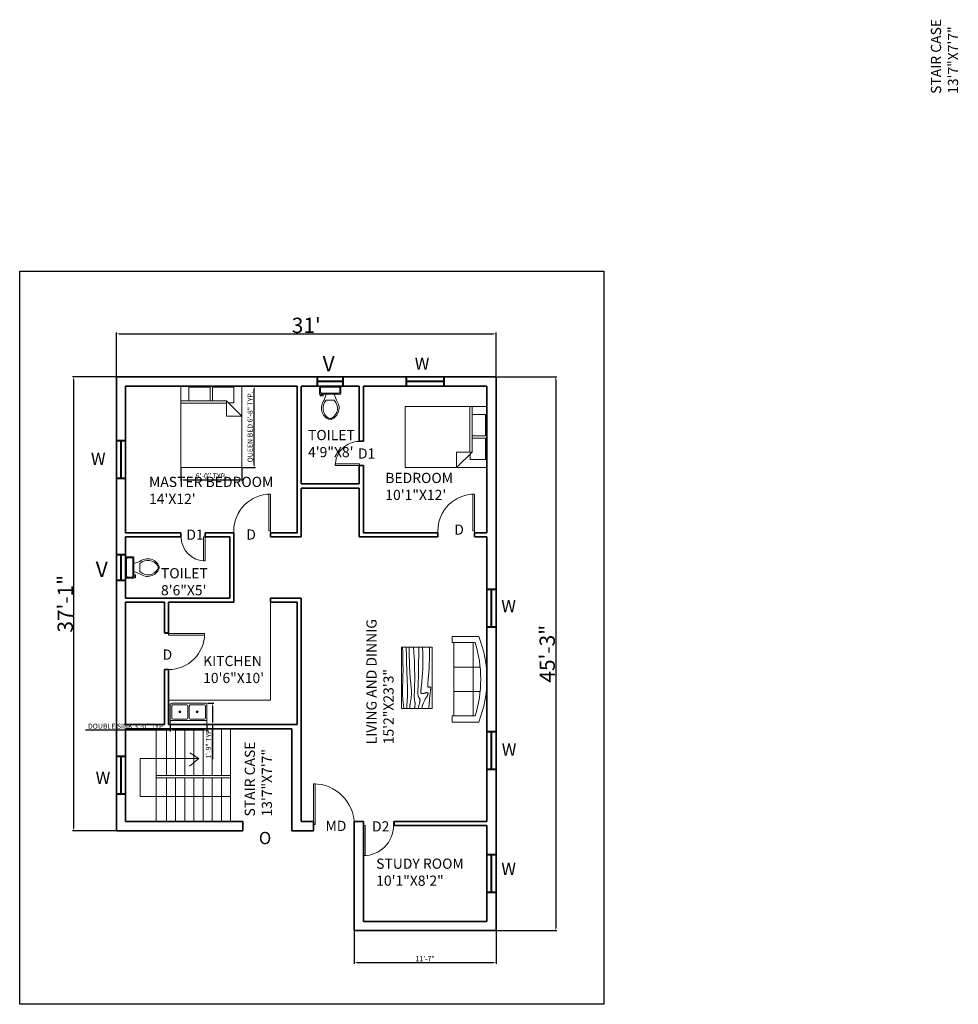
# Model space of a CAD drawing. Units: inches. Extents: x 1662 to 23131, y 1265 to 19127.
# Tile 3 of 26: x 1662 to 2582, y 4561 to 5526. Entities that reach past the tile are written whole.
import ezdxf

# ---------------------------------------------------------------- set-up
doc = ezdxf.new("R2010")
doc.units = ezdxf.units.IN
for name, color, linetype, lineweight in [('A-ANNO-DIMS', 4, 'Continuous', 18), ('A-ANNO-IDEN', 7, 'Continuous', 18), ('A-ANNO-TTLB', 7, 'Continuous', 25), ('A-AREA-IDEN', 7, 'Continuous', 18), ('A-DOOR', 3, 'Continuous', 18), ('A-FLOR-CASE', 8, 'Continuous', 18), ('A-FLOR-FIXT', 9, 'Continuous', 18), ('A-FLOR-STRS', 7, 'Continuous', 18), ('A-FURN', 8, 'Continuous', 18), ('A-GLAZ', 4, 'Continuous', 18), ('A-WALL', 7, 'Continuous', 35)]:
    doc.layers.add(name, color=color, linetype=linetype, lineweight=lineweight)
doc.styles.get("Standard").update_dxf_attribs({"font": 'arial.ttf'})
doc.dimstyles.new('ISO-25', dxfattribs={"dimtxt": 5, "dimasz": 2.5, "dimexe": 1.25, "dimexo": 0.625, "dimtad": 1, "dimlunit": 3, "dimtxsty": 'Standard', "dimcen": 2.5, "dimadec": 0, "dimazin": 0, "dimtfac": 1, "dimtmove": 0, "dimatfit": 3, "dimfxl": 1, "dimarcsym": 0})

# ---------------------------------------------------------------- blocks, each defined once
blk = doc.blocks.new('*U33')
for p, q in [((0, 0), (0, -6)), ((40, 0), (40, -6))]:
    blk.add_line(p, q)
blk.add_lwpolyline([(0, 0), (0, 40), (1.75, 40), (1.75, 0)], close=True)
blk.add_arc((0, 0), 40, 0, 90)
blk = doc.blocks.new('*U25')
for p, q in [((-750, 0), (-750, -100)), ((0, 0), (0, -100))]:
    blk.add_line(p, q)
blk.add_lwpolyline([(0, 0), (0, 750), (-43.75, 750), (-43.75, 0)], close=True)
blk.add_arc((0, 0), 750, 90, 180)
blk = doc.blocks.new('*U34')
for p, q in [((0, 0), (0, -6)), ((-36, 0), (-36, -6))]:
    blk.add_line(p, q)
blk.add_lwpolyline([(0, 0), (0, 36), (-1.75, 36), (-1.75, 0)], close=True)
blk.add_arc((0, 0), 36, 90, 180)
blk = doc.blocks.new('*U35')
for p, q in [((0, 0), (0, -100)), ((600, 0), (600, -100))]:
    blk.add_line(p, q)
blk.add_lwpolyline([(0, 0), (0, 600), (43.75, 600), (43.75, 0)], close=True)
blk.add_arc((0, 0), 600, 0, 90)
blk = doc.blocks.new('*U36')
for p, q in [((-900, 0), (-900, 100)), ((0, 0), (0, 100))]:
    blk.add_line(p, q)
blk.add_lwpolyline([(0, 0), (0, -900), (-43.75, -900), (-43.75, 0)], close=True)
blk.add_arc((0, 0), 900, 180, 270)
blk = doc.blocks.new('Bed - Queen')
for p, q in [((0, -80.00003), (0, 0)), ((0, 0), (59.99999, 0)), ((59.99999, 0), (59.99999, -80.00003)), ((7.99999, -1.2), (28.79998, -1.2)), ((7.99999, -14.4), (7.99999, -1.2)), ((28.79998, -1.2), (28.79998, -14.4)), ((31.19999, -1.2), (51.99999, -1.2)), ((31.19999, -14.4), (31.19999, -1.2)), ((51.99999, -1.2), (51.99999, -16.4)), ((0, -14.4), (44.8, -14.4)), ((44.8, -16.8), (0, -16.8)), ((59.99999, -29.6), (44.8, -14.4)), ((44.8, -14.4), (44.8, -29.6)), ((51.99999, -16.4), (46.79936, -16.4)), ((44.8, -29.6), (59.99999, -29.6)), ((59.99999, -80.00003), (0, -80.00003))]:
    blk.add_line(p, q)
blk = doc.blocks.new('Sink-double - 36 in top')
for p, q in [((-18, -4), (18, -4)), ((-0.75, -18.5), (-0.75, -6.5)), ((0.75, -6.5), (0.75, -18.5))]:
    blk.add_line(p, q)
for points in [[(-16.5, 0), (16.5, 0)], [(-18, -19.5), (-18, -1.5)], [(-16.5, -18.5), (-16.5, -6.5)], [(-15.5, -5.5), (-1.75, -5.5)], [(1.75, -5.5), (15.5, -5.5)], [(16.5, -6.5), (16.5, -18.5)], [(18, -1.5), (18, -19.5)], [(16.5, -21), (-16.5, -21)], [(-1.75, -19.5), (-15.5, -19.5)], [(15.5, -19.5), (1.75, -19.5)]]:
    blk.add_lwpolyline(points)
for centre, radius in [((-8.5, -12.5), 1), ((-8.5, -12.5), 0.5), ((8.5, -12.5), 1), ((8.5, -12.5), 0.5)]:
    blk.add_circle(centre, radius)
for centre, radius, start, end in [((-16.5, -1.5), 1.5, 90, 180), ((16.5, -1.5), 1.5, 0, 90), ((-15.5, -6.5), 1, 90, 180), ((-1.75, -6.5), 1, 0, 90), ((1.75, -6.5), 1, 90, 180), ((15.5, -6.5), 1, 0, 90), ((-15.5, -18.5), 1, 180, 270), ((-1.75, -18.5), 1, 270, 0), ((1.75, -18.5), 1, 180, 270), ((15.5, -18.5), 1, 270, 0), ((-16.5, -19.5), 1.5, 180, 270), ((16.5, -19.5), 1.5, 270, 0)]:
    blk.add_arc(centre, radius, start, end)
blk = doc.blocks.new('Sofa - Roundback 7 ft.')
for p, q in [((-12.00002, -32.4421), (-12.00003, -6.5971)), ((11.99997, -32.4421), (11.99998, -6.5971)), ((-36.000027, -34), (-36.000027, -11.4696)), ((-35.999844, -13.3819), (35.9998, -13.3819)), ((35.99998, -34), (35.99998, -11.4696)), ((-36.000027, -32.4421), (35.99998, -32.4421))]:
    blk.add_line(p, q)
for points in [[(-36.000027, -34), (-42.000027, -34), (-42.000027, -8)], [(41.99998, -8), (41.99998, -34), (35.99998, -34)]]:
    blk.add_lwpolyline(points)
for centre, radius, start, end in [((0, -114.25), 114.25, 68.43141, 111.5686), ((-0.00001, -127.1968), 121.1968, 72.72033, 107.2797)]:
    blk.add_arc(centre, radius, start, end)
blk = doc.blocks.new('Table - Rectangular Woodgrain 60 x 30 in.')
for p, q in [((0, 0), (0, -30)), ((60, 0), (0, 0)), ((60, -30), (60, 0)), ((0, -30), (60, -30))]:
    blk.add_line(p, q)
for points in [[(0, -2.4), (4.8155, -2.418), (9.0302, -2.4688), (12.709, -2.5477), (15.9167, -2.65), (18.7181, -2.7711), (21.1781, -2.9063), (23.3616, -3.0508), (25.3333, -3.2), (27.1477, -3.3495), (28.8172, -3.4958), (30.3437, -3.636), (31.7291, -3.7667), (32.9756, -3.8849), (34.0849, -3.9875), (35.059, -4.0714), (35.9, -4.1334), (36.6114, -4.1711), (37.2041, -4.1854), (37.6906, -4.1779), (38.0833, -4.15), (38.3948, -4.1034), (38.6375, -4.0396), (38.8239, -3.9602), (38.9666, -3.8667), (39.0764, -3.7608), (39.1573, -3.6448), (39.2116, -3.521), (39.2416, -3.3917), (39.2498, -3.2593), (39.2385, -3.1261), (39.21, -2.9944), (39.1666, -2.8667), (39.111, -2.7447), (39.0468, -2.6281), (38.978, -2.5163), (38.9083, -2.4083), (38.8418, -2.3035), (38.7823, -2.201), (38.7337, -2.1001), (38.7, -2), (38.6844, -1.9003), (38.6875, -1.8021), (38.7094, -1.707), (38.75, -1.6167), (38.8094, -1.5326), (38.8875, -1.4563), (38.9844, -1.3893), (39.1, -1.3333), (39.2351, -1.2896), (39.3937, -1.2583), (39.5804, -1.2396), (39.8, -1.2333), (40.057, -1.2396), (40.3562, -1.2583), (40.7023, -1.2896), (41.1, -1.3333), (41.5547, -1.3895), (42.0755, -1.4573), (42.6721, -1.5361), (43.3542, -1.625), (44.1316, -1.7233), (45.014, -1.8302), (46.0114, -1.9449), (47.1333, -2.0667), (48.3862, -2.1947), (49.7625, -2.3281), (51.2513, -2.4663), (52.8416, -2.6083), (54.5226, -2.7535), (56.2833, -2.9011), (58.1127, -3.0501), (60, -3.2)], [(0, -9.2), (6.5759, -9.0858), (11.9385, -9.0365), (16.2527, -9.0418), (19.6833, -9.0917), (22.3952, -9.1759), (24.5531, -9.2844), (26.322, -9.4069), (27.8666, -9.5333), (29.3241, -9.6553), (30.7203, -9.7719), (32.0532, -9.8837), (33.3208, -9.9917), (34.5213, -10.0965), (35.6526, -10.199), (36.7128, -10.2999), (37.7, -10.4), (38.6129, -10.4996), (39.4531, -10.5969), (40.223, -10.6895), (40.925, -10.775), (41.5613, -10.8512), (42.1344, -10.9156), (42.6465, -10.966), (43.1, -11), (43.4976, -11.0158), (43.8437, -11.0136), (44.143, -10.9942), (44.4, -10.9583), (44.6195, -10.9069), (44.8062, -10.8406), (44.9648, -10.7603), (45.1, -10.6667), (45.2155, -10.5598), (45.3114, -10.4365), (45.3871, -10.2929), (45.4416, -10.125), (45.4743, -9.929), (45.4844, -9.7011), (45.4709, -9.4371), (45.4333, -9.1333), (45.3716, -8.7883), (45.2896, -8.4104), (45.1919, -8.0107), (45.0833, -7.6), (44.9685, -7.1893), (44.8521, -6.7896), (44.7388, -6.4117), (44.6333, -6.0667), (44.54, -5.7628), (44.4614, -5.4979), (44.4001, -5.2675), (44.3583, -5.0667), (44.3384, -4.8909), (44.3427, -4.7354), (44.3736, -4.5956), (44.4333, -4.4667), (44.5236, -4.3453), (44.6427, -4.2333), (44.7884, -4.1339), (44.9583, -4.05), (45.1501, -3.9849), (45.3614, -3.9417), (45.59, -3.9234), (45.8333, -3.9333), (46.0915, -3.9749), (46.3734, -4.0531), (46.6906, -4.1736), (47.0542, -4.3417), (47.4756, -4.5629), (47.9661, -4.8427), (48.5372, -5.1866), (49.2, -5.6), (49.9676, -6.0844), (50.8594, -6.625), (51.8965, -7.2031), (53.1, -7.8), (54.491, -8.3969), (56.0906, -8.975), (57.9199, -9.5156), (60, -10)], [(0, -12.8), (5.1847, -12.9322), (9.6213, -13.0323), (13.3963, -13.1059), (16.5958, -13.1583), (19.3063, -13.1952), (21.614, -13.2219), (23.6054, -13.2439), (25.3666, -13.2667), (26.9728, -13.2947), (28.4531, -13.3281), (29.8256, -13.3663), (31.1083, -13.4083), (32.3191, -13.4535), (33.476, -13.501), (34.597, -13.5501), (35.7, -13.6), (36.7984, -13.6497), (37.8875, -13.6979), (38.9578, -13.743), (40, -13.7833), (41.0047, -13.8174), (41.9625, -13.8438), (42.864, -13.8607), (43.7, -13.8667), (44.4631, -13.8604), (45.1552, -13.8417), (45.7801, -13.8104), (46.3416, -13.7667), (46.8439, -13.7104), (47.2906, -13.6417), (47.6858, -13.5604), (48.0333, -13.4667), (48.3375, -13.3608), (48.6042, -13.2448), (48.8396, -13.121), (49.05, -12.9917), (49.2417, -12.8593), (49.4208, -12.7261), (49.5937, -12.5944), (49.7667, -12.4667), (49.9452, -12.3451), (50.1323, -12.2313), (50.3303, -12.1268), (50.5416, -12.0333), (50.7686, -11.9524), (51.0135, -11.8854), (51.2788, -11.8341), (51.5666, -11.8), (51.8785, -11.7843), (52.2116, -11.7865), (52.562, -11.8059), (52.926, -11.8417), (53.2998, -11.8931), (53.6795, -11.9594), (54.0614, -12.0397), (54.4416, -12.1333), (54.8223, -12.2401), (55.2293, -12.3625), (55.6942, -12.5037), (56.2489, -12.6667), (56.9251, -12.8547), (57.7545, -13.0708), (58.7689, -13.3182), (60, -13.6)], [(0, -18), (5.124, -17.7273), (9.6609, -17.5057), (13.6705, -17.3303), (17.2125, -17.1958), (20.3467, -17.0973), (23.1328, -17.0297), (25.6307, -16.9878), (27.9, -16.9667), (29.9928, -16.9617), (31.9302, -16.9703), (33.7254, -16.9907), (35.3917, -17.0208), (36.9423, -17.0588), (38.3906, -17.1026), (39.7499, -17.1503), (41.0333, -17.2), (42.2519, -17.2496), (43.4073, -17.2969), (44.4986, -17.3395), (45.525, -17.375), (46.4858, -17.4012), (47.3802, -17.4156), (48.2074, -17.416), (48.9667, -17.4), (49.6583, -17.3662), (50.2872, -17.3167), (50.8595, -17.2547), (51.3812, -17.1833), (51.8584, -17.1057), (52.2971, -17.025), (52.7034, -16.9443), (53.0833, -16.8667), (53.443, -16.7951), (53.789, -16.7313), (54.128, -16.6768), (54.4666, -16.6334), (54.8115, -16.6024), (55.1693, -16.5854), (55.5465, -16.5841), (55.95, -16.6), (56.3828, -16.6337), (56.8346, -16.6823), (57.2915, -16.7418), (57.7396, -16.8084), (58.165, -16.878), (58.5539, -16.9469), (58.8924, -17.0111), (59.1666, -17.0667), (59.3679, -17.1107), (59.5078, -17.1438), (59.6032, -17.1675), (59.6708, -17.1833), (59.7275, -17.193), (59.7901, -17.1979), (59.8753, -17.1998), (60, -17.2)], [(0, -22.4), (8.0098, -22.2501), (14.4094, -22.1011), (19.4168, -21.9535), (23.25, -21.8083), (26.1269, -21.6663), (28.2656, -21.5281), (29.884, -21.3947), (31.2, -21.2667), (32.3967, -21.1448), (33.5172, -21.0292), (34.5697, -20.9198), (35.5625, -20.8167), (36.5037, -20.7198), (37.4015, -20.6292), (38.2642, -20.5448), (39.1, -20.4667), (39.9164, -20.3951), (40.7187, -20.3313), (41.5117, -20.2768), (42.3, -20.2333), (43.0883, -20.2024), (43.8812, -20.1854), (44.6836, -20.1841), (45.5, -20.2), (46.3328, -20.234), (47.1747, -20.2844), (48.0163, -20.3488), (48.8479, -20.425), (49.66, -20.5106), (50.4429, -20.6031), (51.1872, -20.7004), (51.8833, -20.8), (52.5246, -20.8999), (53.1166, -20.9995), (53.6681, -21.0983), (54.1875, -21.1958), (54.6834, -21.2919), (55.1646, -21.3859), (55.6394, -21.4777), (56.1167, -21.5667), (56.6028, -21.6515), (57.0961, -21.7266), (57.5929, -21.7852), (58.0896, -21.8208), (58.5823, -21.8268), (59.0674, -21.7964), (59.5412, -21.723), (60, -21.6)], [(0, -25.2), (8.6355, -25.0504), (15.7026, -24.9031), (21.4049, -24.7606), (25.9458, -24.625), (29.529, -24.4988), (32.3578, -24.3844), (34.6359, -24.284), (36.5667, -24.2), (38.3213, -24.1341), (39.9417, -24.0854), (41.437, -24.0523), (42.8167, -24.0333), (44.0901, -24.0268), (45.2667, -24.0313), (46.3557, -24.0451), (47.3667, -24.0667), (48.309, -24.0947), (49.1928, -24.1287), (50.0284, -24.168), (50.826, -24.2125), (51.5959, -24.2617), (52.3483, -24.3151), (53.0935, -24.3725), (53.8417, -24.4334), (54.6009, -24.497), (55.3699, -24.561), (56.1454, -24.6226), (56.9239, -24.6792), (57.7021, -24.7279), (58.4764, -24.7662), (59.2435, -24.7911), (60, -24.8)], [(0, -28.8), (5.6867, -28.6681), (10.45, -28.5698), (14.407, -28.5012), (17.675, -28.4584), (20.3711, -28.4374), (22.6125, -28.4344), (24.5164, -28.4455), (26.2, -28.4667), (27.762, -28.4947), (29.2276, -28.5281), (30.6033, -28.5663), (31.8958, -28.6084), (33.1118, -28.6535), (34.2578, -28.7011), (35.3405, -28.7501), (36.3666, -28.8), (37.3443, -28.8497), (38.288, -28.8974), (39.2137, -28.9412), (40.1375, -28.9792), (41.0753, -29.0093), (42.0432, -29.0297), (43.0572, -29.0384), (44.1333, -29.0333), (45.2936, -29.0114), (46.5843, -28.9641), (48.0579, -28.8816), (49.7666, -28.7542), (51.7629, -28.5721), (54.0989, -28.3255), (56.8272, -28.0048), (60, -27.6)]]:
    blk.add_lwpolyline(points)
blk = doc.blocks.new('Toilet - top')
for p, q in [((-10, -8.5), (-8, -8.5)), ((-10, -9.5), (-10, -8.5)), ((-7, -9.5), (-10, -9.5)), ((-8, -8.5), (-8, -8)), ((-7, -8), (-7, -9.5)), ((-4, -8), (-6, -14)), ((4, -8), (6, -14)), ((9.5, -6), (9.5, -2)), ((4, -14), (-4, -14))]:
    blk.add_line(p, q)
blk.add_lwpolyline([(10.5, -8), (10.5, 0), (-10.5, 0), (-10.5, -8)], close=True)
for points in [[(-9.5, -2), (-9.5, -6)], [(8.5, -1), (-8.5, -1)], [(-8.5, -7), (8.5, -7)]]:
    blk.add_lwpolyline(points)
for centre, radius, start, end in [((-8.62, -1.88), 0.884, 81.8699, 188.1301), ((-8.62, -6.12), 0.884, 171.8699, 278.1301), ((8.62, -1.88), 0.884, 351.8699, 98.1301), ((8.62, -6.12), 0.884, 261.8699, 8.1301), ((3.52, -21.58), 12.17, 141.46911, 247.97143), ((4.2, -21.82), 11.33, 136.36773, 238.94682), ((-3.52, -21.58), 12.17, 292.02843, 38.53071), ((-4.2, -21.82), 11.33, 301.05301, 43.63209), ((0, -27.88), 4, 245.73182, 294.26817), ((0, -29), 4, 254.86053, 285.13947)]:
    blk.add_arc(centre, radius, start, end)
blk = doc.blocks.new('*D37')
at = {"layer": 'A-ANNO-DIMS', "color": 0, "lineweight": -2, "transparency": 16777216}
for p, q in [((1757.16, 5176.65), (1757.16, 5219.46)), ((1759.66, 5218.21), (2126.66, 5218.21)), ((2129.16, 5176.65), (2129.16, 5219.46))]:
    blk.add_line(p, q, dxfattribs=at)
at = {"layer": 'A-ANNO-DIMS', "color": 0, "transparency": 16777216}
for points in [[(1759.66, 5218.63), (1759.66, 5217.79), (1757.16, 5218.21)], [(2126.66, 5218.63), (2126.66, 5217.79), (2129.16, 5218.21)]]:
    blk.add_solid(points, dxfattribs=at)
at = {"layer": 'Defpoints', "color": 0, "transparency": 16777216}
for p in [(2129.16, 5218.21), (1757.16, 5176.03), (2129.16, 5176.03)]:
    blk.add_point(p, dxfattribs=at)
at = {"layer": 'A-ANNO-DIMS', "color": 0, "transparency": 16777216, "insert": (1943.16, 5226.5), "char_height": 5, "attachment_point": 5}
blk.add_mtext("{\\H3x;31'}", dxfattribs=at)
blk = doc.blocks.new('*D38')
at = {"layer": 'A-ANNO-DIMS', "color": 0, "lineweight": -2, "transparency": 16777216}
for p, q in [((2129.79, 5176.03), (2188.87, 5176.03)), ((2187.62, 5173.53), (2187.62, 4635.53)), ((2129.79, 4633.03), (2188.87, 4633.03))]:
    blk.add_line(p, q, dxfattribs=at)
at = {"layer": 'A-ANNO-DIMS', "color": 0, "transparency": 16777216}
for points in [[(2187.2, 5173.53), (2188.03, 5173.53), (2187.62, 5176.03)], [(2187.2, 4635.53), (2188.03, 4635.53), (2187.62, 4633.03)]]:
    blk.add_solid(points, dxfattribs=at)
at = {"layer": 'Defpoints', "color": 0, "transparency": 16777216}
for p in [(2129.16, 5176.03), (2129.16, 4633.03), (2187.62, 4633.03)]:
    blk.add_point(p, dxfattribs=at)
at = {"layer": 'A-ANNO-DIMS', "color": 0, "transparency": 16777216, "insert": (2179.33, 4904.53), "char_height": 5, "attachment_point": 5, "rotation": 90}
blk.add_mtext('{\\H3x;45\'-3"}', dxfattribs=at)
blk = doc.blocks.new('*D39')
at = {"layer": 'A-ANNO-DIMS', "color": 0, "lineweight": -2, "transparency": 16777216}
for p, q in [((1756.54, 5176.03), (1714.01, 5176.03)), ((1715.26, 4733.53), (1715.26, 5173.53)), ((1756.54, 4731.03), (1714.01, 4731.03))]:
    blk.add_line(p, q, dxfattribs=at)
at = {"layer": 'A-ANNO-DIMS', "color": 0, "transparency": 16777216}
for points in [[(1714.85, 5173.53), (1715.68, 5173.53), (1715.26, 5176.03)], [(1714.85, 4733.53), (1715.68, 4733.53), (1715.26, 4731.03)]]:
    blk.add_solid(points, dxfattribs=at)
at = {"layer": 'Defpoints', "color": 0, "transparency": 16777216}
for p in [(1715.26, 5176.03), (1757.16, 5176.03), (1757.16, 4731.03)]:
    blk.add_point(p, dxfattribs=at)
at = {"layer": 'A-ANNO-DIMS', "color": 0, "transparency": 16777216, "insert": (1706.97, 4953.53), "char_height": 5, "attachment_point": 5, "rotation": 90}
blk.add_mtext('{\\H3x;37\'-1"}', dxfattribs=at)
blk = doc.blocks.new('WIN-36-J9X1')
for p, q in [((0, 9), (0, 0)), ((1, 9), (1, 0)), ((1, 5), (37, 5)), ((1, 4.5), (37, 4.5)), ((1, 4), (37, 4)), ((37, 9), (37, 0)), ((38, 9), (38, 0))]:
    blk.add_line(p, q)
blk = doc.blocks.new('VENT-24-J9X1')
for p, q in [((0, 9), (0, 0)), ((1, 9), (1, 0)), ((1, 5), (25, 5)), ((1, 4.5), (25, 4.5)), ((1, 4), (25, 4)), ((25, 9), (25, 0)), ((26, 9), (26, 0))]:
    blk.add_line(p, q)
blk = doc.blocks.new('*D157')
at = {"layer": 'A-ANNO-DIMS', "color": 0, "lineweight": -2, "transparency": 16777216}
for p, q in [((1880.79, 5167.03), (1893.41, 5167.03)), ((1892.16, 5089.53), (1892.16, 5164.53)), ((1880.79, 5087.03), (1893.41, 5087.03))]:
    blk.add_line(p, q, dxfattribs=at)
at = {"layer": 'A-ANNO-DIMS', "color": 0, "transparency": 16777216}
for points in [[(1891.74, 5164.53), (1892.58, 5164.53), (1892.16, 5167.03)], [(1891.74, 5089.53), (1892.58, 5089.53), (1892.16, 5087.03)]]:
    blk.add_solid(points, dxfattribs=at)
at = {"layer": 'Defpoints', "color": 0, "transparency": 16777216}
for p in [(1880.16, 5167.03), (1892.16, 5167.03), (1880.16, 5087.03)]:
    blk.add_point(p, dxfattribs=at)
at = {"layer": 'A-ANNO-DIMS', "color": 0, "transparency": 16777216, "insert": (1888.8, 5127.03), "char_height": 5, "attachment_point": 5, "rotation": 90}
blk.add_mtext('QUEEN BED 6\'-8" TYP.', dxfattribs=at)
blk = doc.blocks.new('*D158')
at = {"layer": 'A-ANNO-DIMS', "color": 0, "lineweight": -2, "transparency": 16777216}
for p, q in [((1820.16, 5086.4), (1820.16, 5073.78)), ((1880.16, 5086.4), (1880.16, 5073.78)), ((1822.66, 5075.03), (1877.66, 5075.03))]:
    blk.add_line(p, q, dxfattribs=at)
at = {"layer": 'A-ANNO-DIMS', "color": 0, "transparency": 16777216}
for points in [[(1822.66, 5075.44), (1822.66, 5074.61), (1820.16, 5075.03)], [(1877.66, 5075.44), (1877.66, 5074.61), (1880.16, 5075.03)]]:
    blk.add_solid(points, dxfattribs=at)
at = {"layer": 'Defpoints', "color": 0, "transparency": 16777216}
for p in [(1820.16, 5087.03), (1880.16, 5087.03), (1880.16, 5075.03)]:
    blk.add_point(p, dxfattribs=at)
at = {"layer": 'A-ANNO-DIMS', "color": 0, "transparency": 16777216, "insert": (1850.16, 5078.21), "char_height": 5, "attachment_point": 5}
blk.add_mtext('5\'-0" TYP.', dxfattribs=at)
blk = doc.blocks.new('*D167')
at = {"layer": 'A-ANNO-DIMS', "color": 0, "lineweight": -2, "transparency": 16777216}
for p, q in [((1809.78, 4829.63), (1726.89, 4829.63)), ((1809.78, 4834.4), (1809.78, 4828.38)), ((1843.28, 4829.63), (1812.28, 4829.63)), ((1845.78, 4834.4), (1845.78, 4828.38))]:
    blk.add_line(p, q, dxfattribs=at)
at = {"layer": 'A-ANNO-DIMS', "color": 0, "transparency": 16777216}
for points in [[(1812.28, 4830.04), (1812.28, 4829.21), (1809.78, 4829.63)], [(1843.28, 4830.04), (1843.28, 4829.21), (1845.78, 4829.63)]]:
    blk.add_solid(points, dxfattribs=at)
at = {"layer": 'Defpoints', "color": 0, "transparency": 16777216}
for p in [(1809.78, 4835.03), (1809.78, 4829.63), (1845.78, 4835.03)]:
    blk.add_point(p, dxfattribs=at)
at = {"layer": 'A-ANNO-DIMS', "color": 0, "transparency": 16777216, "insert": (1767.09, 4832.84), "char_height": 5, "attachment_point": 5}
blk.add_mtext('DOUBLE SINK 3\'-0" TYP.', dxfattribs=at)
blk = doc.blocks.new('*D168')
at = {"layer": 'A-ANNO-DIMS', "color": 0, "lineweight": -2, "transparency": 16777216}
for p, q in [((1846.41, 4856.03), (1852.43, 4856.03)), ((1851.18, 4853.53), (1851.18, 4837.53)), ((1846.41, 4835.03), (1852.43, 4835.03)), ((1851.18, 4835.03), (1851.18, 4801.27))]:
    blk.add_line(p, q, dxfattribs=at)
at = {"layer": 'A-ANNO-DIMS', "color": 0, "transparency": 16777216}
for points in [[(1850.76, 4853.53), (1851.6, 4853.53), (1851.18, 4856.03)], [(1850.76, 4837.53), (1851.6, 4837.53), (1851.18, 4835.03)]]:
    blk.add_solid(points, dxfattribs=at)
at = {"layer": 'Defpoints', "color": 0, "transparency": 16777216}
for p in [(1845.78, 4856.03), (1845.78, 4835.03), (1851.18, 4835.03)]:
    blk.add_point(p, dxfattribs=at)
at = {"layer": 'A-ANNO-DIMS', "color": 0, "transparency": 16777216, "insert": (1848, 4816.9), "char_height": 5, "attachment_point": 5, "rotation": 90}
blk.add_mtext('1\'-9" TYP.', dxfattribs=at)
blk = doc.blocks.new('*D204')
at = {"layer": 'A-ANNO-DIMS', "color": 0, "lineweight": -2, "transparency": 16777216}
for p, q in [((1990.16, 4632.4), (1990.16, 4600.53)), ((2129.16, 4632.4), (2129.16, 4600.53)), ((1992.66, 4601.78), (2126.66, 4601.78))]:
    blk.add_line(p, q, dxfattribs=at)
at = {"layer": 'A-ANNO-DIMS', "color": 0, "transparency": 16777216}
for points in [[(1992.66, 4602.19), (1992.66, 4601.36), (1990.16, 4601.78)], [(2126.66, 4602.19), (2126.66, 4601.36), (2129.16, 4601.78)]]:
    blk.add_solid(points, dxfattribs=at)
at = {"layer": 'Defpoints', "color": 0, "transparency": 16777216}
for p in [(1990.16, 4633.03), (2129.16, 4633.03), (2129.16, 4601.78)]:
    blk.add_point(p, dxfattribs=at)
at = {"layer": 'A-ANNO-DIMS', "color": 0, "transparency": 16777216, "insert": (2059.66, 4604.91), "char_height": 5, "attachment_point": 5}
blk.add_mtext('11\'-7"', dxfattribs=at)

msp = doc.modelspace()

# ---------------------------------------------------------------- linework, layer by layer
at = {"layer": 'A-ANNO-TTLB'}
msp.add_lwpolyline([(1662.336, 5279.705), (2234.904, 5279.705), (2234.904, 4560.821), (1662.336, 4560.821)], close=True, dxfattribs=at)
at = {"layer": 'A-FLOR-CASE'}
for p in [(1908.161, 4955.027), (1808.161, 4859.027)]:
    msp.add_line(p, (1908.161, 4859.027), dxfattribs=at)
at = {"layer": 'A-FLOR-STRS'}
for p, q in [((1796.161, 4740.027), (1796.161, 4831.027)), ((1806.057, 4785.027), (1806.057, 4831.027)), ((1815.057, 4785.027), (1815.057, 4831.027)), ((1824.057, 4785.027), (1824.057, 4831.027)), ((1833.057, 4785.027), (1833.057, 4831.027)), ((1842.057, 4785.027), (1842.057, 4831.027)), ((1851.057, 4785.027), (1851.057, 4831.027)), ((1860.057, 4785.027), (1860.057, 4831.027)), ((1869.057, 4740.027), (1869.057, 4831.027)), ((1780.243, 4764.494), (1780.243, 4801.68)), ((1780.243, 4801.68), (1837.824, 4801.68)), ((1837.824, 4801.68), (1828.786, 4794.322)), ((1837.824, 4801.68), (1829.158, 4807.431)), ((1869.057, 4785.027), (1796.161, 4785.027)), ((1869.057, 4783.027), (1796.161, 4783.027)), ((1806.057, 4740.027), (1806.057, 4783.027)), ((1815.057, 4740.027), (1815.057, 4783.027)), ((1824.057, 4740.027), (1824.057, 4783.027)), ((1833.057, 4740.027), (1833.057, 4783.027)), ((1842.057, 4740.027), (1842.057, 4783.027)), ((1851.057, 4740.027), (1851.057, 4783.027)), ((1860.057, 4740.027), (1860.057, 4783.027)), ((1869.057, 4764.494), (1780.243, 4764.494))]:
    msp.add_line(p, q, dxfattribs=at)
at = {"layer": 'A-WALL'}
for p, q in [((1757.161, 5176.027), (2129.161, 5176.027)), ((1757.161, 4731.027), (1757.161, 5176.027)), ((2129.161, 5176.027), (2129.161, 4633.027)), ((1766.161, 5167.027), (1934.161, 5167.027)), ((1766.161, 5023.027), (1766.161, 5167.027)), ((1934.161, 5023.027), (1934.161, 5167.027)), ((1938.161, 5071.027), (1938.161, 5167.027)), ((1938.161, 5167.027), (1995.161, 5167.027)), ((1995.161, 5113.027), (1995.161, 5167.027)), ((1999.161, 5167.027), (2120.161, 5167.027)), ((1999.161, 5113.027), (1999.161, 5167.027)), ((2120.161, 5167.027), (2120.161, 5023.027)), ((2120.161, 5167.027), (2120.161, 5023.027)), ((1995.161, 5113.027), (1999.161, 5113.027)), ((1995.161, 5071.027), (1995.161, 5089.027)), ((1995.161, 5089.027), (1999.161, 5089.027)), ((1999.161, 5023.027), (1999.161, 5089.027)), ((1938.161, 5071.027), (1995.161, 5071.027)), ((1938.161, 5067.027), (1995.161, 5067.027)), ((1938.161, 5019.027), (1938.161, 5067.027)), ((1995.161, 5019.027), (1995.161, 5067.027)), ((1766.161, 5023.027), (1820.161, 5023.027)), ((1820.161, 5019.027), (1820.161, 5023.027)), ((1844.161, 5019.027), (1844.161, 5023.027)), ((1844.161, 5023.027), (1872.161, 5023.027)), ((1872.161, 4955.027), (1872.161, 5023.027)), ((1908.161, 5019.027), (1908.161, 5023.027)), ((1908.161, 5023.027), (1934.161, 5023.027)), ((1999.161, 5023.027), (2072.161, 5023.027)), ((2072.161, 5023.027), (2072.161, 5019.027)), ((2108.161, 5023.027), (2108.161, 5019.027)), ((2108.161, 5023.027), (2120.161, 5023.027)), ((1766.161, 5019.027), (1820.161, 5019.027)), ((1766.161, 4959.027), (1766.161, 5019.027)), ((1844.161, 5019.027), (1868.161, 5019.027)), ((1868.161, 4959.027), (1868.161, 5019.027)), ((1908.161, 5019.027), (1938.161, 5019.027)), ((1995.161, 5019.027), (2072.161, 5019.027)), ((2108.161, 5019.027), (2120.161, 5019.027)), ((2120.161, 5019.027), (2120.161, 4740.027)), ((1766.161, 4959.027), (1868.161, 4959.027)), ((1766.161, 4955.027), (1804.161, 4955.027)), ((1766.161, 4835.027), (1766.161, 4955.027)), ((1804.161, 4925.027), (1804.161, 4955.027)), ((1808.161, 4955.027), (1872.161, 4955.027)), ((1808.161, 4925.027), (1808.161, 4955.027)), ((1908.161, 4959.027), (1938.161, 4959.027)), ((1908.161, 4959.027), (1908.161, 4955.027)), ((1908.161, 4955.027), (1934.161, 4955.027)), ((1934.161, 4835.027), (1934.161, 4955.027)), ((1938.161, 4740.027), (1938.161, 4959.027)), ((1804.161, 4925.027), (1808.161, 4925.027)), ((1804.161, 4835.027), (1804.161, 4889.027)), ((1804.161, 4889.027), (1808.161, 4889.027)), ((1808.161, 4835.027), (1808.161, 4889.027)), ((1766.161, 4835.027), (1804.161, 4835.027)), ((1766.161, 4831.027), (1929.161, 4831.027)), ((1766.161, 4740.027), (1766.161, 4831.027)), ((1808.161, 4835.027), (1934.161, 4835.027)), ((1929.161, 4731.027), (1929.161, 4831.027)), ((1881.161, 4740.027), (1766.161, 4740.027)), ((1881.161, 4740.027), (1881.161, 4731.027)), ((1950.161, 4740.027), (1938.161, 4740.027)), ((1950.161, 4731.027), (1950.161, 4740.027)), ((1990.161, 4633.027), (1990.161, 4740.027)), ((1999.161, 4740.027), (1990.161, 4740.027)), ((1999.161, 4642.027), (1999.161, 4740.027)), ((2120.161, 4740.027), (2029.161, 4740.027)), ((2029.161, 4736.027), (2029.161, 4740.027)), ((1881.161, 4731.027), (1757.161, 4731.027)), ((1938.161, 4731.027), (1929.161, 4731.027)), ((1938.161, 4731.027), (1950.161, 4731.027)), ((2120.161, 4736.027), (2029.161, 4736.027)), ((2120.161, 4736.027), (2120.161, 4642.027)), ((2120.161, 4642.027), (1999.161, 4642.027)), ((2129.161, 4633.027), (1990.161, 4633.027))]:
    msp.add_line(p, q, dxfattribs=at)

# ---------------------------------------------------------------- block references
at = {"layer": 'A-DOOR', "xscale": 0.0393700787401575, "yscale": 0.0393700787401575, "zscale": 0.0393700787401575}
for name, p, rotation in [('*U35', (1995.224, 5089.027), 89.99999999999996), ('*U35', (1844.161, 5019.09), 180), ('*U36', (1808.161, 4924.46), 89.99999999999996), ('*U25', (1999.161, 4736.09), 180)]:
    msp.add_blockref(name, p, dxfattribs=dict(at, rotation=rotation))
at = {"layer": 'A-DOOR'}
for name, p in [('*U34', (1908.161, 5025.027)), ('*U34', (2108.161, 5025.027)), ('*U33', (1950.161, 4737.027))]:
    msp.add_blockref(name, p, dxfattribs=at)
at = {"layer": 'A-FLOR-FIXT'}
msp.add_blockref('Toilet - top', (1966.661, 5167.027), dxfattribs=at)
for name, p, rotation in [('Toilet - top', (1766.161, 4989.027), 89.99999999999999), ('Sink-double - 36 in top', (1827.78, 4835.027), 180)]:
    msp.add_blockref(name, p, dxfattribs=dict(at, rotation=rotation))
at = {"layer": 'A-FURN'}
msp.add_blockref('Bed - Queen', (1820.161, 5167.027), dxfattribs=at)
for name, p, rotation in [('Bed - Queen', (2120.161, 5147.088), 270), ('Sofa - Roundback 7 ft.', (2120.161, 4879.527), 269.9999999999999), ('Table - Rectangular Woodgrain 60 x 30 in.', (2066.425, 4910.887), 270)]:
    msp.add_blockref(name, p, dxfattribs=dict(at, rotation=rotation))
at = {"layer": 'A-GLAZ'}
for name, p in [('VENT-24-J9X1', (1953.661, 5167.027)), ('WIN-36-J9X1', (2040.661, 5167.027))]:
    msp.add_blockref(name, p, dxfattribs=at)
at = {"layer": 'A-GLAZ', "rotation": 90}
for name, p in [('WIN-36-J9X1', (1766.161, 5076.028)), ('VENT-24-J9X1', (1766.161, 4976.028)), ('WIN-36-J9X1', (2129.161, 4930.278)), ('WIN-36-J9X1', (2129.161, 4790.778)), ('WIN-36-J9X1', (1766.161, 4766.528)), ('WIN-36-J9X1', (2129.161, 4670.028))]:
    msp.add_blockref(name, p, dxfattribs=at)

# ---------------------------------------------------------------- texts
at = {"layer": 'A-ANNO-IDEN', "attachment_point": 1}
for s, width, heights, insert, char_height in [('V', 1142.59551, [20], (1959.191, 5196.444), 15), ('W', 471.52273, [28.462], (2049.484, 5194.989), 12), ('W', 471.52273, [28.462], (1732.137, 5101.727), 12), ('D1', 1142.59551, [20], (1993.836, 5105.871), 10), ('D', 1142.59551, [0], (2088.245, 5031.228), 10), ('D1', 1142.59551, [20], (1825.708, 5026.295), 10), ('D', 1142.59551, [0], (1884.432, 5026.43), 10), ('V', 1142.59551, [20], (1736.893, 4994.747), 15), ('W', 471.52273, [28.462], (2134.286, 4957.279), 12), ('D', 1142.59551, [0], (1802.391, 4908.705), 10), ('W', 471.52273, [28.462], (2134.763, 4816.61), 12), ('W', 471.52273, [28.462], (1736.771, 4788.954), 12), ('MD', 1142.59551, [0], (1962.016, 4740.733), 10), ('D2', 1142.59551, [20], (2007.664, 4740.258), 10), ('O', 471.52273, [28.462], (1896.721, 4729.832), 12), ('W', 471.52273, [28.462], (2134.303, 4699.702), 12)]:
    msp.add_mtext_dynamic_manual_height_columns(s, width=width, gutter_width=12.5, heights=heights, dxfattribs=dict(at, insert=insert, char_height=char_height))
at = {"layer": 'A-AREA-IDEN', "char_height": 10, "attachment_point": 1, "rotation": 90}
for s, insert in [('STAIR CASE\\P13\'7"X7\'7"', (2555.322, 5453.471)), ('LIVING AND DINNIG\\P15\'2"X23\'3"', (2002.105, 4815.793)), ('STAIR CASE\\P13\'7"X7\'7"', (1882.883, 4744.949))]:
    msp.add_mtext_dynamic_manual_height_columns(s, width=1142.59551, gutter_width=12.5, heights=[277.772], dxfattribs=dict(at, insert=insert))
at = {"layer": 'A-AREA-IDEN', "char_height": 10, "attachment_point": 1}
for s, insert in [('TOILET \\P4\'9"X8\'', (1944.887, 5123.932)), ("MASTER BEDROOM\\P14'X12'", (1789.095, 5078.04)), ('BEDROOM\\P10\'1"X12\'', (2020.635, 5081.922)), ('TOILET \\P8\'6"X5\'', (1800.776, 4988.467)), ('KITCHEN\\P10\'6"X10\'', (1842.094, 4902.438)), ('STUDY ROOM\\P10\'1"X8\'2"', (2011.681, 4703.695))]:
    msp.add_mtext_dynamic_manual_height_columns(s, width=1142.59551, gutter_width=12.5, heights=[277.772], dxfattribs=dict(at, insert=insert))

# ---------------------------------------------------------------- dimensions: what is measured, and where the dimension line sits
at = {"layer": 'A-ANNO-DIMS'}
for base, p1, p2, text, override, picture, middle in [((2129.161, 5218.21), (1757.161, 5176.027), (2129.161, 5176.027), '{\\H3x;<>}', {"dimclrd": 0, "dimclre": 0, "dimclrt": 0}, '*D37', (1943.161, 5226.499)), ((1880.161, 5075.027), (1820.161, 5087.027), (1880.161, 5087.027), '<> TYP.', {"dimdec": 1, "dimlfac": 1, "dimrnd": 0, "dimzin": 1, "dimdsep": 46, "dimlunit": 4, "dimfrac": 2}, '*D158', (1850.161, 5078.205))]:
    dim = msp.add_linear_dim(base=base, p1=p1, p2=p2, text=text, dimstyle='ISO-25', override=override, dxfattribs=at)
    dim.commit()
    dim.dimension.update_dxf_attribs({"geometry": picture, "text_midpoint": middle})
for base, p1, p2, angle, text, override, picture, middle in [((1715.262, 5176.027), (1757.161, 4731.027), (1757.161, 5176.027), 90, '{\\H3x;<>}', {"dimclrd": 0, "dimclre": 0, "dimclrt": 0}, '*D39', (1706.973, 4953.527)), ((2187.615, 4633.027), (2129.161, 5176.027), (2129.161, 4633.027), 90, '{\\H3x;<>}', {"dimclrd": 0, "dimclre": 0, "dimclrt": 0}, '*D38', (2179.327, 4904.527)), ((1892.161, 5167.027), (1880.161, 5087.027), (1880.161, 5167.027), 90, 'QUEEN BED <> TYP.', {"dimdec": 1, "dimlfac": 1, "dimrnd": 0, "dimzin": 1, "dimdsep": 46, "dimlunit": 4, "dimfrac": 2}, '*D157', (1888.797, 5127.027)), ((1851.18, 4835.027), (1845.78, 4856.027), (1845.78, 4835.027), 270, '<> TYP.', {"dimdec": 1, "dimlfac": 1, "dimrnd": 0, "dimzin": 1, "dimdsep": 46, "dimlunit": 4, "dimfrac": 2}, '*D168', (1848.002, 4816.899)), ((1809.78, 4829.627), (1845.78, 4835.027), (1809.78, 4835.027), 180, 'DOUBLE SINK <> TYP.', {"dimdec": 1, "dimlfac": 1, "dimrnd": 0, "dimzin": 1, "dimdsep": 46, "dimlunit": 4, "dimfrac": 2}, '*D167', (1767.087, 4832.841))]:
    dim = msp.add_linear_dim(base=base, p1=p1, p2=p2, angle=angle, text=text, dimstyle='ISO-25', override=override, dxfattribs=at)
    dim.commit()
    dim.dimension.update_dxf_attribs({"geometry": picture, "text_midpoint": middle})
dim = msp.add_linear_dim(base=(2129.161, 4601.777), p1=(1990.161, 4633.027), p2=(2129.161, 4633.027), dimstyle='ISO-25', override={"dimdec": 1, "dimlfac": 1, "dimrnd": 0, "dimzin": 1, "dimdsep": 46, "dimlunit": 4, "dimfrac": 2}, dxfattribs=at)
dim.commit()
dim.dimension.update_dxf_attribs({"geometry": '*D204', "text_midpoint": (2059.661, 4604.912)})

doc.saveas('drawing.dxf')
